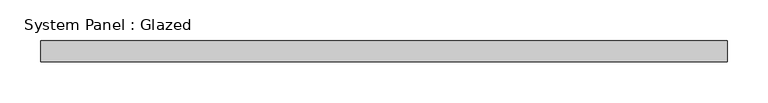
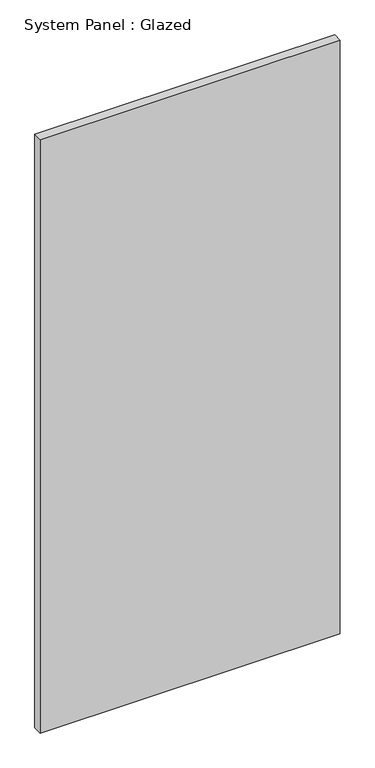
"""IFC4 building model written with IfcOpenShell, lengths in millimetres: plate geometry, System Panel : Glazed."""

from ifc_helpers import new_model, si_unit, origin, origin_with_axes, place, context, project, spatial, polyline, outline, extrude, source, transform, mapped, element, save


def system_panel_glazed_1b7191b4(model_context):
    return source(origin(), model_context, "Body", "SweptSolid", [
        extrude(outline(polyline([(419.1, 19.05), (-419.1, 19.05), (-419.1, 44.45), (419.1, 44.45), (419.1, 19.05)])), origin_with_axes(), (0.0, 0.0, 1.0), 1752.6),
    ])


if __name__ == "__main__":
    model = new_model("IFC4")
    model_context = context("Model", 3, world=origin())
    ifc_project = project(units=[si_unit("LENGTHUNIT", "METRE", prefix="MILLI")], contexts=[model_context])
    site = spatial("IfcSite", under=ifc_project)
    building = spatial("IfcBuilding", under=site)
    placement = place(None, origin())
    system_panel_glazed_shape = system_panel_glazed_1b7191b4(model_context)
    element("IfcPlate", 1, ObjectType="System Panel : Glazed", at=placement, inside=building, context=model_context, shape_type="MappedRepresentation", body=[
        mapped(system_panel_glazed_shape, transform((0.0, 0.0, 0.0), x_axis=(1.0, 0.0, 0.0), y_axis=(0.0, 1.0, 0.0), z_axis=(0.0, 0.0, 1.0))),
    ])
    save(model, "model.ifc")

# Revit data of these elements
# Type "System Panel : Glazed"
#   Construction Type Id = "GSP4R"
#   Analytic Construction = "1/8 in Pilkington single glazing"
#   Visual Light Transmittance = 0.9
#   Solar Heat Gain Coefficient = 0.86
#   Heat Transfer Coefficient (U) = 1.18115 BTU/(h·ft²·°F)
#   Define Thermal Properties by = 1
# Element 1 (IfcPlate, "System Panel : Glazed")
#   Materials on its faces: "Glass"
# Materials
#   "Glass": class "Glass", colour RGB 0 128 192, transparency 0.75, Description = "Soda Lime Glass", Cost = 0
